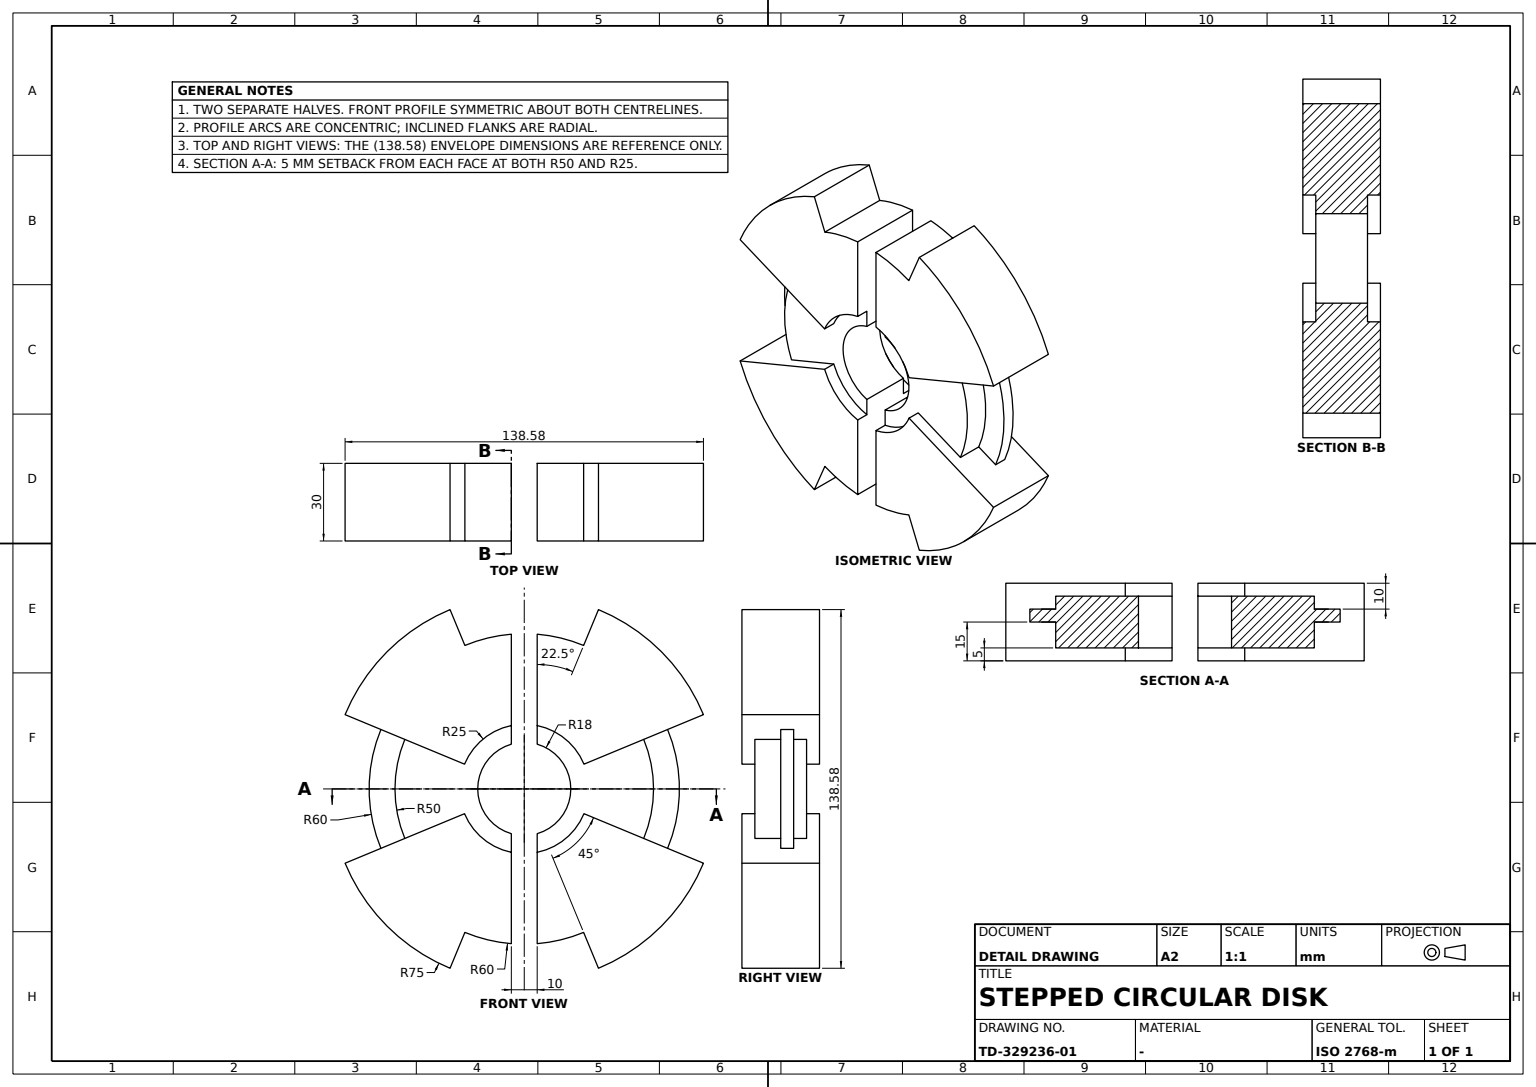
CATIA V5 part; units mm, degrees
sketch "Sketch1" plane through (0, 0, 0) normal (0, 0, 1) x (1, 0, 0)
  circle A0 centre (0, 0) radius 60
  dimension "radius A0" = 60
extrude "Pad1" add sketch "Sketch1" against normal blind 5
sketch "Sketch2" plane through (0, 0, 0) normal (0, 0, 1) x (1, 0, 0)
  circle A0 centre (0, 0) radius 50
  dimension "radius A0" = 50
extrude "Pad2" add sketch "Sketch2" along normal mid plane 20
sketch "Sketch3" plane through (0, 0, 0) normal (0, 0, 1) x (1, 0, 0)
  arc A0 (69.291, 28.7013) -> (-69.291, 28.7013) centre (0, 0) ccw
  arc A1 (23.097, 9.5671) -> (-23.097, 9.5671) centre (0, 0) ccw
  line L0 (-110, 0) -> (140, 0) construction
  point P0 (-110, 0)
  line L1 (78.3938, 32.4718) -> (-91.4594, -37.8837) construction
  point P1 (78.3938, 32.4718)
  point P2 (-91.4594, -37.8837)
  point P3 (91.4594, -37.8837)
  point P4 (-78.3938, 32.4718)
  line L2 (-78.3938, 32.4718) -> (91.4594, -37.8837) construction
  line L3 (23.097, 9.5671) -> (69.291, 28.7013)
  point P5 (23.097, 9.5671)
  point P6 (69.291, 28.7013)
  point P7 (23.097, -9.5671)
  point P8 (69.291, 28.7013)
  point P9 (69.291, -28.7013)
  point P10 (23.097, 9.5671)
  point P11 (23.097, -9.5671)
  arc A2 (-69.291, -28.7013) -> (69.291, -28.7013) centre (0, 0) ccw
  point P12 (-69.291, -28.7013)
  point P13 (-69.291, 28.7013)
  point P14 (-23.097, 9.5671)
  arc A3 (-23.097, -9.5671) -> (23.097, -9.5671) centre (0, 0) ccw
  point P15 (-23.097, -9.5671)
  point P16 (69.291, -28.7013)
  point P17 (23.097, -9.5671)
  line L4 (23.097, -9.5671) -> (69.291, -28.7013)
  point P18 (-69.291, -28.7013)
  point P19 (-23.097, -9.5671)
  line L5 (-23.097, -9.5671) -> (-69.291, -28.7013)
  point P20 (-69.291, 28.7013)
  point P21 (-23.097, 9.5671)
  line L6 (-23.097, 9.5671) -> (-69.291, 28.7013)
  dimension "radius A0" = 75
  dimension "radius A1" = 25
  dimension "angle L1 L0" = 22.5
  constraint coincidence P0 x-axis
  constraint coincidence L1 origin
  constraint coincidence P5 A1
  constraint coincidence P5 L1
  constraint coincidence P6 A0
  constraint coincidence P7 A1
  constraint coincidence P7 L2
  constraint coincidence L3 P8
  constraint coincidence L2 P9
  constraint coincidence L1 P10
  constraint coincidence L2 P11
  constraint coincidence L1 P12
  constraint coincidence A0 A2
  constraint coincidence L2 P13
  constraint coincidence A1 A3
  constraint coincidence P8 P6
  constraint coincidence P13 P20
  constraint coincidence P10 P5
  constraint coincidence P14 P21
  constraint coincidence P9 P16
  constraint coincidence P11 P17
  constraint coincidence P12 P18
  constraint coincidence P15 P19
  constraint horizontal L0 x-axis
  constraint symmetry P2 P3 y-axis
  constraint symmetry P1 P4 y-axis
  constraint symmetry L1 L2 y-axis
  constraint symmetry P6 P16 L0
  constraint symmetry P5 P17 L0
  constraint symmetry L3 L4 L0
  constraint symmetry P16 P18 y-axis
  constraint symmetry P17 P19 y-axis
  constraint symmetry L4 L5 y-axis
  constraint symmetry P6 P20 y-axis
  constraint symmetry P5 P21 y-axis
  constraint symmetry L3 L6 y-axis
  constraint parallelism L3 L1
extrude "Pad3" add sketch "Sketch3" along normal mid plane 30
sketch "Sketch4" plane through (0, 0, 15) normal (0, 0, 1) x (1, 0, 0)
  arc A0 (-28.7013, -69.291) -> (28.7013, -69.291) centre (0, 0) ccw
  arc A1 (22.961, 55.4328) -> (5, 59.7913) centre (0, 0) ccw
  line L0 (35.2817, 85.1775) -> (-35.2817, -85.1775) construction
  point P0 (35.2817, 85.1775)
  point P1 (-35.2817, -85.1775)
  point P2 (35.2817, -85.1775)
  point P3 (-35.2817, 85.1775)
  line L1 (-35.2817, 85.1775) -> (35.2817, -85.1775) construction
  line L2 (22.961, 55.4328) -> (28.7013, 69.291)
  point P4 (22.961, 55.4328)
  point P5 (28.7013, 69.291)
  point P6 (-28.7013, 69.291)
  point P7 (-22.961, 55.4328)
  line L3 (-22.961, 55.4328) -> (-28.7013, 69.291)
  point P8 (28.7013, -69.291)
  point P9 (22.961, -55.4328)
  line L4 (22.961, -55.4328) -> (28.7013, -69.291)
  point P10 (-28.7013, -69.291)
  point P11 (-22.961, -55.4328)
  line L5 (-22.961, -55.4328) -> (-28.7013, -69.291)
  point P12 (-28.7013, 69.291)
  point P13 (-28.7013, -69.291)
  point P14 (28.7013, -69.291)
  arc A2 (28.7013, 69.291) -> (-28.7013, 69.291) centre (0, 0) ccw
  point P15 (28.7013, 69.291)
  point P16 (22.961, 55.4328)
  point P17 (-22.961, 55.4328)
  arc A3 (-22.961, -55.4328) -> (-5, -59.7913) centre (0, 0) ccw
  point P18 (-22.961, -55.4328)
  arc A4 (5, -59.7913) -> (22.961, -55.4328) centre (0, 0) ccw
  arc A5 (-5, 59.7913) -> (-22.961, 55.4328) centre (0, 0) ccw
  line L6 (5, 59.7913) -> (5, -59.7913)
  line L7 (-5, 59.7913) -> (-5, -59.7913)
  dimension "radius A0" = 75
  dimension "radius A1" = 60
  dimension "angle y axis L0" = 22.5
  dimension "distance y axis L6" = 5
  dimension "distance y axis L7" = 5
  constraint coincidence L0 origin
  constraint coincidence P4 A1
  constraint coincidence P4 L0
  constraint coincidence P5 A0
  constraint coincidence P5 L0
  constraint coincidence L1 P12
  constraint coincidence L0 P13
  constraint coincidence L1 P14
  constraint coincidence L0 P15
  constraint coincidence A0 A2
  constraint coincidence L0 P16
  constraint coincidence L1 P17
  constraint coincidence L0 P18
  constraint coincidence A1 A3
  constraint coincidence A3 A4
  constraint coincidence A1 A5
  constraint coincidence P13 P10
  constraint coincidence P14 P8
  constraint coincidence P16 P4
  constraint coincidence P5 P15
  constraint coincidence P6 P12
  constraint coincidence P7 P17
  constraint coincidence P11 P18
  constraint symmetry P1 P2 y-axis
  constraint symmetry P0 P3 y-axis
  constraint symmetry L0 L1 y-axis
  constraint symmetry P5 P6 y-axis
  constraint symmetry P4 P7 y-axis
  constraint symmetry L2 L3 y-axis
  constraint symmetry P5 P8 x-axis
  constraint symmetry P4 P9 x-axis
  constraint symmetry L2 L4 x-axis
  constraint symmetry P6 P10 x-axis
  constraint symmetry P7 P11 x-axis
  constraint symmetry L3 L5 x-axis
  constraint vertical L6 y-axis
  constraint vertical L7 y-axis
extrude "Pocket1" cut sketch "Sketch4" against normal blind 15
sketch "Pocket2 profile" plane through (0, 0, 0) normal (0, 0, 1) x (1, 0, 0)
  arc A0 (-28.7013, -69.291) -> (28.7013, -69.291) centre (0, 0) ccw
  line L0 (22.961, -55.4328) -> (28.7013, -69.291)
  arc A1 (5, -59.7913) -> (22.961, -55.4328) centre (0, 0) ccw
  line L1 (5, 59.7913) -> (5, -59.7913)
  arc A2 (22.961, 55.4328) -> (5, 59.7913) centre (0, 0) ccw
  line L2 (22.961, 55.4328) -> (28.7013, 69.291)
  arc A3 (28.7013, 69.291) -> (-28.7013, 69.291) centre (0, 0) ccw
  line L3 (-22.961, 55.4328) -> (-28.7013, 69.291)
  arc A4 (-5, 59.7913) -> (-22.961, 55.4328) centre (0, 0) ccw
  line L4 (-5, 59.7913) -> (-5, -59.7913)
  arc A5 (-22.961, -55.4328) -> (-5, -59.7913) centre (0, 0) ccw
  line L5 (-22.961, -55.4328) -> (-28.7013, -69.291)
extrude "Pocket2" cut sketch "Pocket2 profile" against normal through all and the other way through all
sketch "Sketch5" plane through (0, 0, 0) normal (0, 0, 1) x (1, 0, 0)
  circle A0 centre (0, 0) radius 18
  dimension "radius A0" = 18
extrude "Pocket3" cut sketch "Sketch5" along normal mid plane 30
